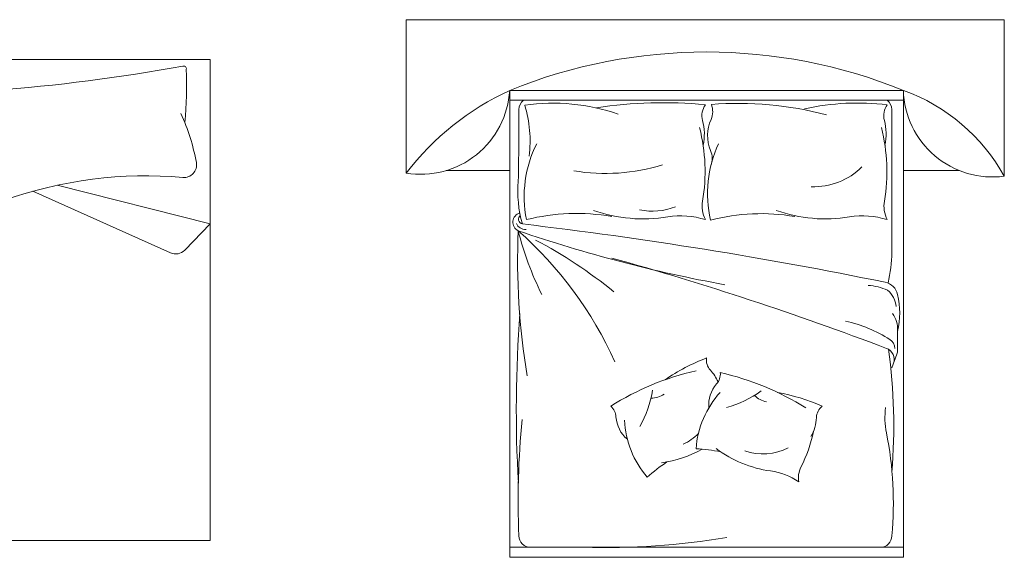
# Model space of a CAD drawing. Units: inches. Extents: x 1994 to 3075, y 3517 to 3950.
# Tile 47 of 58: x 1994.6046 to 1994.7701, y 3553.7966 to 3553.8869. Entities that reach past the tile are written whole.
import ezdxf

# ---------------------------------------------------------------- set-up
doc = ezdxf.new("R2010")
doc.units = ezdxf.units.IN
doc.layers.add('A-FURN-REFR', color=8, linetype='Continuous', lineweight=13)

msp = doc.modelspace()

# ---------------------------------------------------------------- linework, layer by layer
at = {"layer": 'A-FURN-REFR'}
for p, q in [((1994.669579926378, 3553.886876991775), (1994.669579926378, 3553.861116444467)), ((1994.770060054451, 3553.886876991762), (1994.669579926378, 3553.886876991762)), ((1994.770060054451, 3553.886876991762), (1994.770060054451, 3553.860604701765)), ((1994.636645156601, 3553.880219755423), (1994.596260242865, 3553.880219755423)), ((1994.636645156601, 3553.880219755423), (1994.596260242865, 3553.880219755423)), ((1994.636645156601, 3553.799449927951), (1994.636645156601, 3553.880219755423)), ((1994.686956049541, 3553.875013338293), (1994.753105865942, 3553.875013338279)), ((1994.686956049541, 3553.875013338293), (1994.686956049525, 3553.796606350029)), ((1994.753105865942, 3553.875013338279), (1994.753105865926, 3553.796606350015)), ((1994.753105865942, 3553.860604701765), (1994.753105865942, 3553.875013338279)), ((1994.686956049541, 3553.873340137054), (1994.753105865942, 3553.873340137041)), ((1994.751160283102, 3553.847832768839), (1994.751160283106, 3553.871783670773)), ((1994.636645156601, 3553.799449927951), (1994.636645156601, 3553.864775123905)), ((1994.676295856829, 3553.861542943156), (1994.686956049541, 3553.861542943156)), ((1994.753105865942, 3553.861542943142), (1994.762506594516, 3553.861542943142)), ((1994.606831479664, 3553.858065865062), (1994.629975887107, 3553.84773133204)), ((1994.61095246929, 3553.859078122546), (1994.636656011856, 3553.852591011417)), ((1994.632354937459, 3553.848187382655), (1994.636645156601, 3553.852593751088)), ((1994.752133074516, 3553.831385131824), (1994.752133074516, 3553.835202958813)), ((1994.752012868837, 3553.830711863078), (1994.751160283097, 3553.828400318778)), ((1994.596260242865, 3553.799449927951), (1994.636645156601, 3553.799449927951)), ((1994.596260242865, 3553.799449927951), (1994.636645156601, 3553.799449927951)), ((1994.686956049525, 3553.798279551267), (1994.753105865927, 3553.798279551254)), ((1994.686956049525, 3553.796606350029), (1994.753105865926, 3553.796606350015))]:
    msp.add_line(p, q, dxfattribs=at)
for centre, radius, start, end in [((1994.720030957744, 3553.79333837511), 0.0881178140957525, 67.95413287556839, 112.0458671276888), ((1994.578229990593, 3554.173819251654), 0.2996159645214513, 274.1894661393186, 280.345956739574), ((1994.63218847432, 3553.87865222054), 0.0004482907065646, 350.157018905503, 109.5558986651033), ((1994.56374144405, 3553.876029527558), 0.0689357559366832, 354.6669486061241, 2.116631318036676), ((1994.672013535948, 3553.875885209347), 0.0149679280998906, 260.6428391444751, 356.6606718254233), ((1994.706655884585, 3553.832569794828), 0.0467924981438534, 114.8979987522044, 142.4055122176543), ((1994.76806772771, 3553.875439441593), 0.0149679280998906, 181.6313026200066, 277.6491353005932), ((1994.742348592341, 3553.845176545523), 0.031716764294517, 29.10655736921449, 70.17388055115411), ((1994.690458098644, 3553.871783670785), 0.0019455828353276, 126.8698976337993, 179.9999999880876), ((1994.6941987666, 3553.839063779813), 0.0338061826761343, 71.0292396466785, 98.01463022582239), ((1994.670302804081, 3553.866602123392), 0.0200804373013914, 352.4610811587552, 17.19907473199907), ((1994.712701940969, 3553.800990034885), 0.071952262989263, 84.30946080187233, 98.94135126792816), ((1994.722362449769, 3553.870777823127), 0.0031075126812102, 144.3787648229011, 195.1987658355305), ((1994.717862302794, 3553.871458612669), 0.0032028341489732, 335.7877323280015, 21.71237864400314), ((1994.725450233601, 3553.816325645749), 0.0565064023996118, 74.89247536308716, 94.681970907379), ((1994.745429930372, 3553.831416409507), 0.0414680575843914, 83.14136388124066, 102.4247502365447), ((1994.752908100284, 3553.87077782312), 0.0031075126812102, 144.3787648229011, 195.1987658355305), ((1994.749214700271, 3553.871783670774), 0.0019455828353276, 359.9999999880876, 53.13010234330246), ((1994.599639144952, 3553.856579485091), 0.0352435291682938, 10.28821543962675, 24.3977020455474), ((1994.150894123828, 3553.87094266847), 0.5376190497749752, 358.8114973710085, 0.0896283401223897), ((1994.711068031897, 3553.867709458949), 0.0085962787467616, 347.311957921453, 15.19876583553051), ((1994.72678134222, 3553.867447941822), 0.0065764677133891, 155.7877323280015, 202.8808293159797), ((1994.741613682412, 3553.867709458943), 0.0085962787467616, 347.311957921453, 15.19876583553051), ((1994.689928429448, 3553.861395612989), 0.0298558147000044, 350.3711224665587, 14.25995084780135), ((1994.720474079963, 3553.861395612983), 0.0298558147000044, 350.3711224665587, 14.25995084780135), ((1994.709151392715, 3553.857168820011), 0.0197598411462801, 153.3318705081994, 191.2891230798232), ((1994.740048484023, 3553.857684712184), 0.0198519972069101, 155.1179531461462, 192.9861889591517), ((1994.717644973931, 3553.863592190669), 0.0033401870886801, 339.0160855821216, 22.88082931597971), ((1994.632233849104, 3553.862496021546), 0.0021161969121165, 265.0123902482592, 10.28821543962675), ((1994.703074195901, 3553.893285330661), 0.0322267158934928, 260.4320326468418, 287.2701993260345), ((1994.738042407286, 3553.870276393172), 0.0114567055564695, 267.8294752673963, 315.0098308273483), ((1994.625862123298, 3553.789485019043), 0.0711723108928985, 85.01239024825922, 109.5152363667157), ((1994.708370398146, 3553.858063531221), 0.0200474922626186, 175.0553728283678, 195.8557099358243), ((1994.724289333978, 3553.855566085884), 0.004996088352876, 170.3711224665586, 206.9649370961853), ((1994.754834984493, 3553.855566085878), 0.004996088352876, 170.3711224665586, 206.9649370961853), ((1994.689105675149, 3553.852891276032), 0.0016105685091622, 106.3004786234319, 243.938180591863), ((1994.698199112393, 3553.819760440479), 0.034582210914614, 80.14382640862489, 104.1008515969175), ((1994.709428472714, 3553.878831958021), 0.0254057342932298, 250.6572032486362, 279.2500666033769), ((1994.711013781629, 3553.864715795235), 0.009989213432703, 257.148031947205, 292.3825063085086), ((1994.740036878674, 3553.878065339755), 0.0246390736856652, 250.3559327023518, 279.3925899659531), ((1994.689252922745, 3553.853381735724), 0.0008128892221172, 129.3957755051945, 258.1255955891823), ((1994.715725931064, 3553.840374301304), 0.0135641447689492, 72.35976010254194, 99.39258996595309), ((1994.72919672886, 3553.820614117447), 0.0336972432594088, 80.32657587842615, 104.5973118255227), ((1994.746271581578, 3553.840374301297), 0.0135641447689492, 72.35976010254194, 99.39258996595309), ((1994.689573678189, 3553.85327775552), 0.0016095821071006, 202.6051908922757, 274.4988817166678), ((1994.804914869829, 3553.846345157776), 0.1166283141987217, 177.4940716817132, 189.5094068679036), ((1994.644927705726, 3553.802390851098), 0.065543355857517, 24.38326925012849, 48.45324971012612), ((1994.765134501669, 3554.074263626768), 0.2356625857026807, 250.9968676421653, 259.7279623061984), ((1994.740837217981, 3553.864703272706), 0.0540893550839264, 194.1893851607317, 206.3095844034524), ((1994.602641109589, 3553.119808568226), 0.737858914858732, 78.47703152821846, 83.27200853442297), ((1994.652946657325, 3553.777464711659), 0.0819509525067612, 51.03759283326017, 62.08562985249065), ((1994.630838710283, 3553.849663642972), 0.0021161969121165, 245.9380924250792, 315.7651815658561), ((1994.726442986614, 3553.848164407364), 0.0247195212287987, 347.0890423172248, 359.2312934508153), ((1994.560841168105, 3553.333368817847), 0.5331120127502642, 69.18683318772709, 74.4079909335134), ((1994.749488045842, 3553.840127661344), 0.0027238159694586, 12.88269036848606, 78.38686031445394), ((1994.74659779785, 3553.833156738125), 0.0091331594194461, 65.03385580996276, 86.4640048798947), ((1994.747950806645, 3553.838390732927), 0.0039416012902181, 4.684898432501862, 50.59840531545589), ((1994.738663190353, 3553.837651880079), 0.013828183994568, 346.9286456497866, 12.88269036848606), ((1994.904883703301, 3553.821271170561), 0.2168115609509192, 175.697202442643, 183.2229785434103), ((1994.737812579001, 3553.812347354746), 0.0245737753138132, 58.01122975656369, 76.86512646864662), ((1994.747945886496, 3553.834954317942), 0.0041945638393764, 356.601689895136, 37.73019638534235), ((1994.749948106053, 3553.831703483653), 0.001728440251783, 359.0101027185217, 59.29760239232226), ((1994.749623550305, 3553.829856164811), 0.0019455828353276, 339.7541012352643, 70.67241641354788), ((1994.658311651859, 3553.818763307456), 0.0931787946855045, 355.1752823324409, 7.876466900264919), ((1994.75018749168, 3553.831385131824), 0.0019455828353276, 339.7541012352643, 359.9999999880876), ((1994.75018749168, 3553.831385131824), 0.0019455828353276, 339.7541012352643, 359.9999999880876), ((1994.73185390568, 3553.79907991238), 0.0331744460675131, 110.8823159298724, 124.5017030449515), ((1994.722491420182, 3553.829734438404), 0.0024860101449681, 172.1197168712306, 222.9397178838013), ((1994.728164843498, 3553.783811376605), 0.0452051219196895, 102.6334274117044, 122.4229229559715), ((1994.715637016628, 3553.823356073289), 0.0068770229974093, 23.06813348750885, 42.93971788380129), ((1994.719792798772, 3553.827410977903), 0.0025622673191785, 318.5500264992555, 4.47467281546091), ((1994.712520150304, 3553.783486840405), 0.0452051219196895, 57.654769534688, 77.44426507900442), ((1994.692723878579, 3553.827714336612), 0.0185020874209313, 330.3454935344927, 350.5126648384766), ((1994.725656734062, 3553.822232126712), 0.0052611741707113, 138.5500264992554, 185.6431234876255), ((1994.702032361964, 3553.812892067487), 0.0238846517600035, 33.43324039147294, 33.44627937316185), ((1994.710705923161, 3553.827061090805), 0.0037447944261748, 269.8428349959402, 305.6126069524626), ((1994.734108104389, 3553.813654218166), 0.0158815977655281, 137.8802473178581, 175.7484831308576), ((1994.718482785567, 3553.839593692682), 0.0185020874209313, 285.3668356574626, 305.534006961408), ((1994.730741004199, 3553.826421117634), 0.0037447944261748, 224.8641771190216, 260.6339490755313), ((1994.725922145521, 3553.791679757388), 0.0331744460675131, 65.90365805271031, 79.52304516794653), ((1994.702261813606, 3553.820022622276), 0.0025622673191785, 3.528684376760561, 49.45333069284981), ((1994.717761857705, 3553.821452027693), 0.0026721496709441, 5.54816698551457, 5.64312348762549), ((1994.740967350621, 3553.819981663754), 0.0024860101449681, 127.1410589942614, 177.9610600071594), ((1994.762979426067, 3553.82004969527), 0.0129749866847535, 172.4746658505032, 191.3425348756069), ((1994.829675551054, 3553.806207029259), 0.1412897221787423, 174.5126540947314, 182.4265021937969), ((1994.710070422713, 3553.820504141291), 0.0052611741707113, 183.5286843767605, 230.6217813648581), ((1994.722111907118, 3553.820410179915), 0.0158815977655281, 182.8589051950864, 220.7271410079812), ((1994.731610245426, 3553.820314788354), 0.0068770229974093, 330.0742520930186, 357.9610600071594), ((1994.705037230854, 3553.814371881765), 0.0026721496709441, 50.52682486300737, 50.62178136485808), ((1994.712152504643, 3553.823843717561), 0.0091653644451756, 295.570427315862, 315.3772891878563), ((1994.714590306359, 3553.822529222853), 0.0238846517600035, 333.1334166378931, 348.4676214958053), ((1994.691881258739, 3553.805787982537), 0.0595394659951302, 354.6389628949611, 11.34253487560691), ((1994.709676310877, 3553.83197984082), 0.0197112589485322, 278.0968847510169, 299.1559945636731), ((1994.717028337525, 3553.787902424095), 0.0269577946075271, 78.44814032526723, 87.35960599722004), ((1994.733489472928, 3553.830628269021), 0.0197112589485322, 233.1182268740081, 262.1548841372723), ((1994.729490093863, 3553.823122737438), 0.0091653644451756, 250.591769438949, 297.77212499891), ((1994.728232674515, 3553.790121410702), 0.0269577946075271, 123.4267982025162, 132.338263874535), ((1994.739462332165, 3553.809929158329), 0.0039968706823008, 153.1334166378931, 189.7272312675173), ((1994.729317813953, 3553.800351739538), 0.0108513158151594, 55.1220542741174, 82.15488413760009), ((1994.690458098629, 3553.800225134102), 0.0019455828353276, 179.9999999880876, 269.9999999880876), ((1994.703000575131, 3553.92236545861), 0.1241401229318277, 268.3066004926072, 279.4831521227457), ((1994.749214700257, 3553.80022513409), 0.0019455828353276, 269.9999999880876, 359.9999999880876)]:
    msp.add_arc(centre, radius, start, end, dxfattribs=at)

doc.saveas('drawing.dxf')
